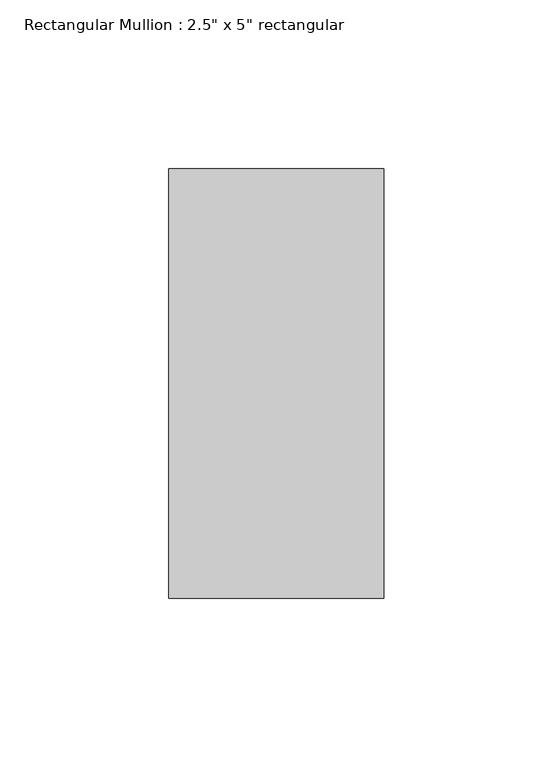
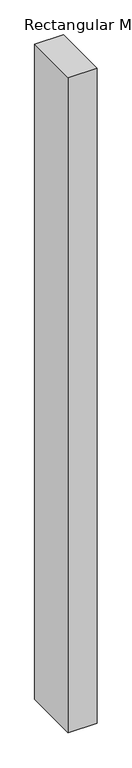
"""IFC4 building model written with IfcOpenShell, lengths in millimetres: member geometry."""

from ifc_helpers import new_model, si_unit, frame, origin, place, context, project, spatial, polyline, outline, extrude, source, transform, mapped, element, save


def member_eeb7212f(model_context):
    return source(origin(), model_context, "Body", "SweptSolid", [
        extrude(outline(polyline([(0.0, 63.5), (0.0, -63.5), (-63.5, -63.5), (-63.5, 63.5), (0.0, 63.5)])), frame((0.0, 0.0, -1521.9137173), z_axis=(0.0, 0.0, 1.0), x_axis=(1.0, 0.0, 0.0)), (0.0, 0.0, 1.0), 1521.9137173),
    ])


if __name__ == "__main__":
    model = new_model("IFC4")
    model_context = context("Model", 3, world=origin())
    ifc_project = project(units=[si_unit("LENGTHUNIT", "METRE", prefix="MILLI")], contexts=[model_context])
    site = spatial("IfcSite", under=ifc_project)
    building = spatial("IfcBuilding", under=site)
    placement = place(None, origin())
    member_shape = member_eeb7212f(model_context)
    element("IfcMember", 1, ObjectType="Rectangular Mullion : 2.5\" x 5\" rectangular", at=placement, inside=building, context=model_context, shape_type="MappedRepresentation", body=[
        mapped(member_shape, transform((0.0, 0.0, 0.0), x_axis=(1.0, 0.0, 0.0), y_axis=(0.0, 1.0, 0.0), z_axis=(0.0, 0.0, 1.0))),
    ])
    save(model, "model.ifc")

# Revit data of these elements
# Type "Rectangular Mullion : 2.5\" x 5\" rectangular"
#   built-in parameter 1007304 = 0.416667 (stored number, unit not read)
#   built-in parameter 1007301 = 0.104167 (stored number, unit not read)
#   built-in parameter 1007300 = 0.104167 (stored number, unit not read)
# Element 1 (IfcMember, "Rectangular Mullion : 2.5\" x 5\" rectangular")
#   Materials on its faces: "Aluminum"
# Materials
#   "Aluminum": class "Metal", colour RGB 247 247 247, transparency 0, Description = "Aluminum 6061", Cost = 0
